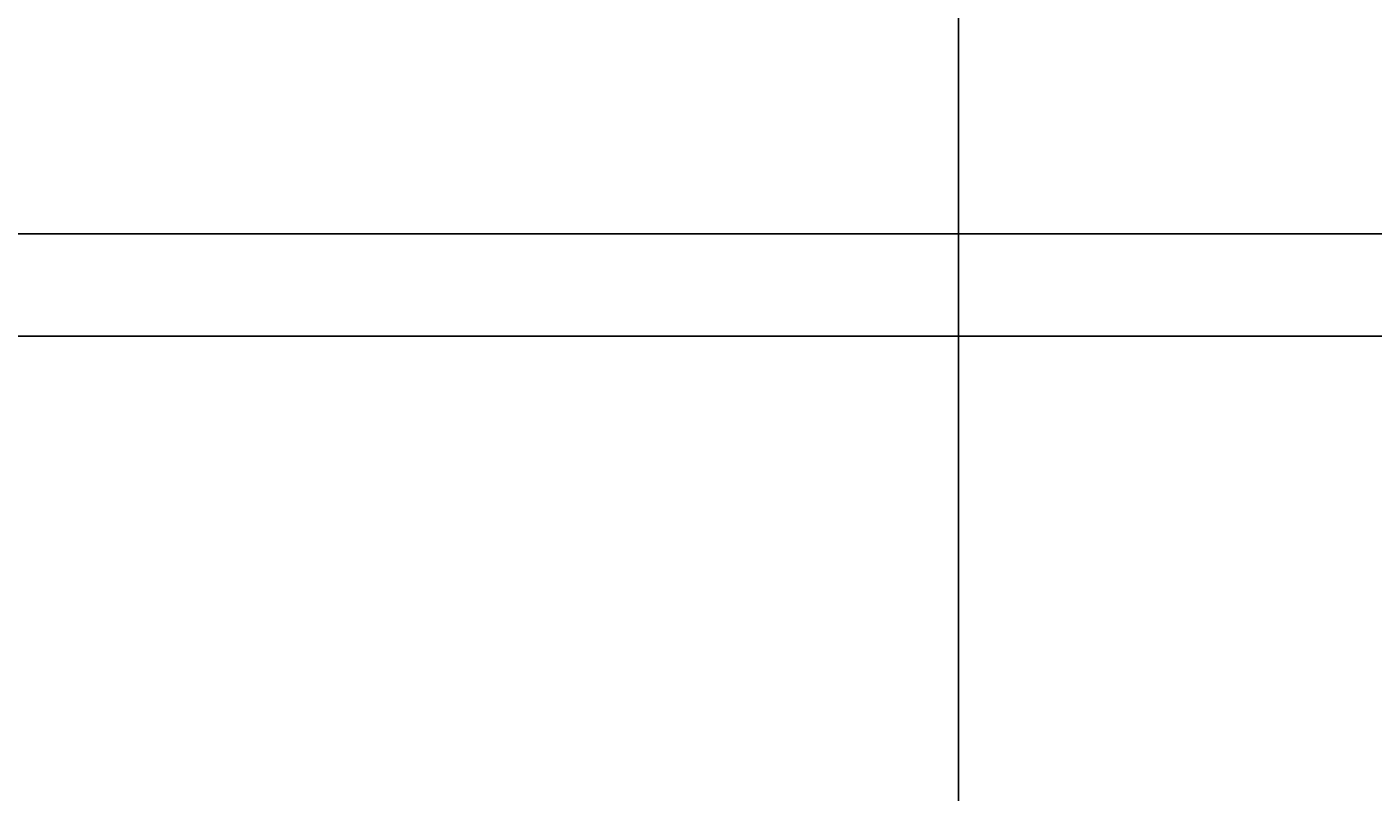
# Model space of a CAD drawing. Units: inches. Extents: x 35362 to 73946, y 43607 to 67532.
# Tile 67 of 134: x 48170 to 48464, y 48798 to 48965. Entities that reach past the tile are written whole.
import ezdxf

# ---------------------------------------------------------------- set-up
doc = ezdxf.new("R2010")
doc.units = ezdxf.units.IN
doc.header["$MEASUREMENT"] = 0
doc.layers.add('A-ANNO-DIMS', color=2, linetype='Continuous', lineweight=18)
doc.styles.get("Standard").update_dxf_attribs({"font": 'arial.ttf'})
doc.dimstyles.get("Standard").update_dxf_attribs({"dimtxt": 0.18, "dimasz": 0.18, "dimexe": 0.18, "dimexo": 0.0625, "dimgap": 0.09, "dimtad": 0, "dimtih": 1, "dimtoh": 1, "dimdec": 4, "dimzin": 0, "dimdsep": 46, "dimtxsty": 'Standard', "dimcen": 0.09, "dimadec": 0, "dimazin": 0, "dimtfac": 1, "dimtdec": 4, "dimtofl": 0, "dimtmove": 0, "dimatfit": 3, "dimfxl": 1, "dimtolj": 1, "dimtzin": 0, "dimarcsym": 0})

# ---------------------------------------------------------------- blocks, each defined once
blk = doc.blocks.new('*D11')
at = {"layer": 'A-ANNO-DIMS', "color": 0, "lineweight": -2, "transparency": 16777216}
for p, q in [((47978.66, 56028.77), (47978.66, 43606.68)), ((53109.76, 56028.77), (53109.76, 43606.68)), ((47978.84, 43606.86), (50543.87, 43606.86)), ((53109.58, 43606.86), (50544.55, 43606.86))]:
    blk.add_line(p, q, dxfattribs=at)
at = {"layer": 'A-ANNO-DIMS', "color": 0, "transparency": 16777216}
for points in [[(47978.84, 43606.89), (47978.84, 43606.83), (47978.66, 43606.86)], [(53109.58, 43606.89), (53109.58, 43606.83), (53109.76, 43606.86)]]:
    blk.add_solid(points, dxfattribs=at)
at = {"layer": 'Defpoints', "color": 0, "transparency": 16777216}
for p in [(47978.66, 56028.84), (53109.76, 56028.84), (53109.76, 43606.86)]:
    blk.add_point(p, dxfattribs=at)
at = {"layer": 'A-ANNO-DIMS', "color": 0, "transparency": 16777216, "insert": (50544.21, 43606.86), "char_height": 0.18, "attachment_point": 5}
blk.add_mtext('\\A1;5131', dxfattribs=at)
blk = doc.blocks.new('*D13')
at = {"layer": 'A-ANNO-DIMS', "color": 0, "lineweight": -2, "transparency": 16777216}
for p, q in [((48373.49, 51694.02), (48373.49, 43606.68)), ((51029.04, 51694.02), (51029.04, 43606.68)), ((48373.67, 43606.86), (49700.8, 43606.86)), ((51028.86, 43606.86), (49701.73, 43606.86))]:
    blk.add_line(p, q, dxfattribs=at)
at = {"layer": 'A-ANNO-DIMS', "color": 0, "transparency": 16777216}
for points in [[(48373.67, 43606.89), (48373.67, 43606.83), (48373.49, 43606.86)], [(51028.86, 43606.89), (51028.86, 43606.83), (51029.04, 43606.86)]]:
    blk.add_solid(points, dxfattribs=at)
at = {"layer": 'Defpoints', "color": 0, "transparency": 16777216}
for p in [(48373.49, 51694.09), (51029.04, 51694.09), (51029.04, 43606.86)]:
    blk.add_point(p, dxfattribs=at)
at = {"layer": 'A-ANNO-DIMS', "color": 0, "transparency": 16777216, "insert": (49701.27, 43606.86), "char_height": 0.18, "attachment_point": 5}
blk.add_mtext('\\A1;2655.6', dxfattribs=at)
blk = doc.blocks.new('*D27')
at = {"layer": 'A-ANNO-DIMS', "color": 0, "lineweight": -2, "transparency": 16777216}
for p, q in [((47978.66, 56028.77), (47978.66, 43606.68)), ((48373.49, 53428.96), (48373.49, 43606.68)), ((47978.84, 43606.86), (48175.68, 43606.86)), ((48373.31, 43606.86), (48176.47, 43606.86))]:
    blk.add_line(p, q, dxfattribs=at)
at = {"layer": 'A-ANNO-DIMS', "color": 0, "transparency": 16777216}
for points in [[(47978.84, 43606.89), (47978.84, 43606.83), (47978.66, 43606.86)], [(48373.31, 43606.89), (48373.31, 43606.83), (48373.49, 43606.86)]]:
    blk.add_solid(points, dxfattribs=at)
at = {"layer": 'Defpoints', "color": 0, "transparency": 16777216}
for p in [(47978.66, 56028.84), (48373.49, 53429.02), (48373.49, 43606.86)]:
    blk.add_point(p, dxfattribs=at)
at = {"layer": 'A-ANNO-DIMS', "color": 0, "transparency": 16777216, "insert": (48176.08, 43606.86), "char_height": 0.18, "attachment_point": 5}
blk.add_mtext('\\A1;394.8', dxfattribs=at)
blk = doc.blocks.new('*D67')
at = {"layer": 'A-ANNO-DIMS', "color": 0, "lineweight": -2, "transparency": 16777216}
for p, q in [((56873.54, 53351.53), (35361.77, 53351.53)), ((35361.95, 53351.35), (35361.95, 49400.89)), ((35361.95, 45450.07), (35361.95, 49400.53)), ((53793.58, 45449.89), (35361.77, 45449.89))]:
    blk.add_line(p, q, dxfattribs=at)
at = {"layer": 'A-ANNO-DIMS', "color": 0, "transparency": 16777216}
for points in [[(35361.92, 53351.35), (35361.98, 53351.35), (35361.95, 53351.53)], [(35361.92, 45450.07), (35361.98, 45450.07), (35361.95, 45449.89)]]:
    blk.add_solid(points, dxfattribs=at)
at = {"layer": 'Defpoints', "color": 0, "transparency": 16777216}
for p in [(35361.95, 53351.53), (56873.6, 53351.53), (53793.64, 45449.89)]:
    blk.add_point(p, dxfattribs=at)
at = {"layer": 'A-ANNO-DIMS', "color": 0, "transparency": 16777216, "insert": (35361.95, 49400.71), "char_height": 0.18, "attachment_point": 5}
blk.add_mtext('\\A1;7901.6', dxfattribs=at)
blk = doc.blocks.new('*D86')
at = {"layer": 'A-ANNO-DIMS', "color": 0, "lineweight": -2, "transparency": 16777216}
for p, q in [((51285.53, 49320.08), (35361.77, 49320.08)), ((35361.95, 49319.9), (35361.95, 49120.26)), ((35361.95, 48920.26), (35361.95, 49119.9)), ((51285.53, 48920.08), (35361.77, 48920.08))]:
    blk.add_line(p, q, dxfattribs=at)
at = {"layer": 'A-ANNO-DIMS', "color": 0, "transparency": 16777216}
for points in [[(35361.92, 49319.9), (35361.98, 49319.9), (35361.95, 49320.08)], [(35361.92, 48920.26), (35361.98, 48920.26), (35361.95, 48920.08)]]:
    blk.add_solid(points, dxfattribs=at)
at = {"layer": 'Defpoints', "color": 0, "transparency": 16777216}
for p in [(35361.95, 49320.08), (51285.59, 49320.08), (51285.59, 48920.08)]:
    blk.add_point(p, dxfattribs=at)
at = {"layer": 'A-ANNO-DIMS', "color": 0, "transparency": 16777216, "insert": (35361.95, 49120.08), "char_height": 0.18, "attachment_point": 5}
blk.add_mtext('\\A1;400.0', dxfattribs=at)
blk = doc.blocks.new('*D89')
at = {"layer": 'A-ANNO-DIMS', "color": 0, "lineweight": -2, "transparency": 16777216}
for p, q in [((53707.72, 48897.74), (35361.77, 48897.74)), ((35361.95, 48897.56), (35361.95, 48303.16)), ((35361.95, 47708.4), (35361.95, 48302.8)), ((53707.72, 47708.22), (35361.77, 47708.22))]:
    blk.add_line(p, q, dxfattribs=at)
at = {"layer": 'A-ANNO-DIMS', "color": 0, "transparency": 16777216}
for points in [[(35361.92, 48897.56), (35361.98, 48897.56), (35361.95, 48897.74)], [(35361.92, 47708.4), (35361.98, 47708.4), (35361.95, 47708.22)]]:
    blk.add_solid(points, dxfattribs=at)
at = {"layer": 'Defpoints', "color": 0, "transparency": 16777216}
for p in [(53707.78, 48897.74), (35361.95, 47708.22), (53707.78, 47708.22)]:
    blk.add_point(p, dxfattribs=at)
at = {"layer": 'A-ANNO-DIMS', "color": 0, "transparency": 16777216, "insert": (35361.95, 48302.98), "char_height": 0.18, "attachment_point": 5}
blk.add_mtext('\\A1;1189.5', dxfattribs=at)

msp = doc.modelspace()

# ---------------------------------------------------------------- dimensions: what is measured, and where the dimension line sits
at = {"layer": 'A-ANNO-DIMS'}
for base, p1, p2, override, picture, middle in [((53109.76, 43606.859), (47978.665, 56028.836), (53109.76, 56028.836), {"dimdec": 0, "dimlfac": 1, "dimrnd": 0, "dimzin": 0, "dimdsep": 46, "dimlunit": 2}, '*D11', (50544.212, 43606.859)), ((48373.492, 43606.859), (47978.665, 56028.836), (48373.492, 53429.019), {"dimdec": 1, "dimlfac": 1, "dimrnd": 0, "dimzin": 0, "dimdsep": 46, "dimlunit": 2}, '*D27', (48176.078, 43606.859)), ((51029.043, 43606.859), (48373.492, 51694.087), (51029.043, 51694.087), {"dimdec": 1, "dimlfac": 1, "dimrnd": 0, "dimzin": 0, "dimdsep": 46, "dimlunit": 2}, '*D13', (49701.267, 43606.859))]:
    dim = msp.add_linear_dim(base=base, p1=p1, p2=p2, dimstyle='Standard', override=override, dxfattribs=at)
    dim.commit()
    dim.dimension.update_dxf_attribs({"geometry": picture, "text_midpoint": middle})
for base, p1, p2, picture, middle in [((35361.949, 53351.529), (53793.638, 45449.894), (56873.602, 53351.529), '*D67', (35361.949, 49400.712)), ((35361.949, 49320.079), (51285.595, 48920.079), (51285.595, 49320.079), '*D86', (35361.949, 49120.079)), ((35361.949, 47708.216), (53707.781, 48897.738), (53707.781, 47708.216), '*D89', (35361.949, 48302.977))]:
    dim = msp.add_linear_dim(base=base, p1=p1, p2=p2, angle=90, dimstyle='Standard', override={"dimdec": 1, "dimlfac": 1, "dimrnd": 0, "dimzin": 0, "dimdsep": 46, "dimlunit": 2}, dxfattribs=at)
    dim.commit()
    dim.dimension.update_dxf_attribs({"geometry": picture, "text_midpoint": middle})

doc.saveas('drawing.dxf')
